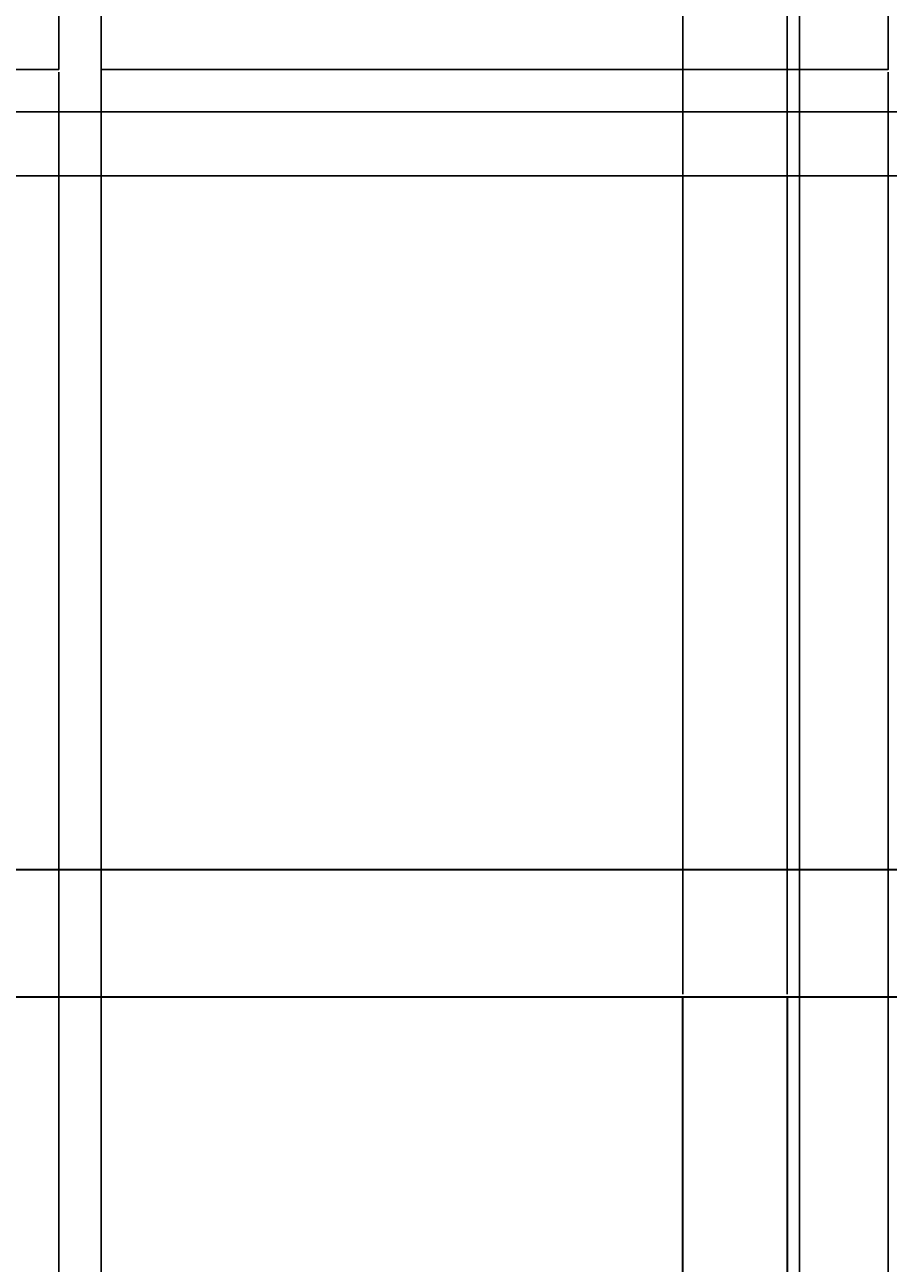
# Model space of a CAD drawing. Units: inches. Extents: x -6 to 289, y -8 to 323.
# Tile 54 of 107: x 146 to 166, y 153 to 182. Entities that reach past the tile are written whole.
import ezdxf

# ---------------------------------------------------------------- set-up
doc = ezdxf.new("R2010")
doc.units = ezdxf.units.IN
doc.header["$MEASUREMENT"] = 0
for name, color, linetype, lineweight in [('A-ANNO-DIMS', 2, 'Continuous', 18), ('A-ELEV', 7, 'Continuous', 35), ('A-ELEV-PATT', 8, 'Continuous', 13), ('A-GLAZ', 4, 'Continuous', 25)]:
    doc.layers.add(name, color=color, linetype=linetype, lineweight=lineweight)
doc.styles.get("Standard").update_dxf_attribs({"font": 'arial.ttf'})
doc.dimstyles.get("Standard").update_dxf_attribs({"dimtxt": 0.18, "dimasz": 0.18, "dimexe": 0.18, "dimexo": 0.0625, "dimgap": 0.09, "dimtad": 0, "dimtih": 1, "dimtoh": 1, "dimdec": 4, "dimzin": 0, "dimdsep": 46, "dimtxsty": 'Standard', "dimcen": 0.09, "dimadec": 0, "dimazin": 0, "dimtfac": 1, "dimtdec": 4, "dimtofl": 0, "dimtmove": 0, "dimatfit": 3, "dimfxl": 1, "dimtolj": 1, "dimtzin": 0, "dimarcsym": 0})

# ---------------------------------------------------------------- blocks, each defined once
blk = doc.blocks.new('*U4')
for p, q in [((21, 1.5), (21, 46.5)), ((21, 1.5), (1.5, 1.5)), ((40.5, 1.5), (21, 1.5))]:
    blk.add_line(p, q)
blk.add_lwpolyline([(0, 0), (0, 48), (42, 48), (42, 0)], close=True)
for points in [[(20, 45.5), (20, 2.5), (2.5, 2.5), (2.5, 45.5), (20, 45.5)], [(21, 45.5), (39.5, 45.5), (39.5, 2.5), (21, 2.5)]]:
    blk.add_lwpolyline(points)
blk = doc.blocks.new('*D24')
at = {"layer": 'A-ANNO-DIMS', "color": 0, "lineweight": -2, "transparency": 16777216}
for p, q in [((126.946, 178.654), (288.653, 178.654)), ((288.473, 178.474), (288.473, 159.153)), ((288.473, 139.469), (288.473, 158.789)), ((259.226, 139.289), (288.653, 139.289))]:
    blk.add_line(p, q, dxfattribs=at)
at = {"layer": 'A-ANNO-DIMS', "color": 0, "transparency": 16777216}
for points in [[(288.443, 178.474), (288.503, 178.474), (288.473, 178.654)], [(288.443, 139.469), (288.503, 139.469), (288.473, 139.289)]]:
    blk.add_solid(points, dxfattribs=at)
at = {"layer": 'Defpoints', "color": 0, "transparency": 16777216}
for p in [(126.883, 178.654), (288.473, 178.654), (259.164, 139.289)]:
    blk.add_point(p, dxfattribs=at)
at = {"layer": 'A-ANNO-DIMS', "color": 0, "transparency": 16777216, "insert": (288.473, 158.971), "char_height": 0.18, "attachment_point": 5}
blk.add_mtext('\\A1;39.365', dxfattribs=at)
blk = doc.blocks.new('*D25')
at = {"layer": 'A-ANNO-DIMS', "color": 0, "lineweight": -2, "transparency": 16777216}
for p, q in [((126.946, 226.654), (288.653, 226.654)), ((288.473, 226.474), (288.473, 202.836)), ((288.473, 178.834), (288.473, 202.472)), ((126.946, 178.654), (288.653, 178.654))]:
    blk.add_line(p, q, dxfattribs=at)
at = {"layer": 'A-ANNO-DIMS', "color": 0, "transparency": 16777216}
for points in [[(288.443, 226.474), (288.503, 226.474), (288.473, 226.654)], [(288.443, 178.834), (288.503, 178.834), (288.473, 178.654)]]:
    blk.add_solid(points, dxfattribs=at)
at = {"layer": 'Defpoints', "color": 0, "transparency": 16777216}
for p in [(126.883, 226.654), (288.473, 226.654), (126.883, 178.654)]:
    blk.add_point(p, dxfattribs=at)
at = {"layer": 'A-ANNO-DIMS', "color": 0, "transparency": 16777216, "insert": (288.473, 202.654), "char_height": 0.18, "attachment_point": 5}
blk.add_mtext('\\A1;48', dxfattribs=at)
blk = doc.blocks.new('*D30')
at = {"layer": 'A-ANNO-DIMS', "color": 0, "lineweight": -2, "transparency": 16777216}
for p, q in [((129.383, 181.092), (129.383, -8.391)), ((146.883, 181.092), (146.883, -8.391)), ((129.563, -8.211), (137.817, -8.211)), ((146.703, -8.211), (138.449, -8.211))]:
    blk.add_line(p, q, dxfattribs=at)
at = {"layer": 'A-ANNO-DIMS', "color": 0, "transparency": 16777216}
for points in [[(129.563, -8.181), (129.563, -8.241), (129.383, -8.211)], [(146.703, -8.181), (146.703, -8.241), (146.883, -8.211)]]:
    blk.add_solid(points, dxfattribs=at)
at = {"layer": 'Defpoints', "color": 0, "transparency": 16777216}
for p in [(129.383, 181.154), (146.883, 181.154), (146.883, -8.211)]:
    blk.add_point(p, dxfattribs=at)
at = {"layer": 'A-ANNO-DIMS', "color": 0, "transparency": 16777216, "insert": (138.133, -8.211), "char_height": 0.18, "attachment_point": 5}
blk.add_mtext('\\A1;17.5', dxfattribs=at)
blk = doc.blocks.new('*D31')
at = {"layer": 'A-ANNO-DIMS', "color": 0, "lineweight": -2, "transparency": 16777216}
for p, q in [((146.883, 181.092), (146.883, -8.391)), ((147.883, 181.092), (147.883, -8.391)), ((147.063, -8.211), (147.26, -8.211)), ((147.703, -8.211), (147.507, -8.211))]:
    blk.add_line(p, q, dxfattribs=at)
at = {"layer": 'A-ANNO-DIMS', "color": 0, "transparency": 16777216}
for points in [[(147.063, -8.181), (147.063, -8.241), (146.883, -8.211)], [(147.703, -8.181), (147.703, -8.241), (147.883, -8.211)]]:
    blk.add_solid(points, dxfattribs=at)
at = {"layer": 'Defpoints', "color": 0, "transparency": 16777216}
for p in [(146.883, 181.154), (147.883, 181.154), (147.883, -8.211)]:
    blk.add_point(p, dxfattribs=at)
at = {"layer": 'A-ANNO-DIMS', "color": 0, "transparency": 16777216, "insert": (147.383, -8.211), "char_height": 0.18, "attachment_point": 5}
blk.add_mtext('\\A1;1', dxfattribs=at)
blk = doc.blocks.new('*D32')
at = {"layer": 'A-ANNO-DIMS', "color": 0, "lineweight": -2, "transparency": 16777216}
for p, q in [((147.883, 181.092), (147.883, -8.391)), ((166.383, 181.092), (166.383, -8.391)), ((148.063, -8.211), (156.817, -8.211)), ((166.203, -8.211), (157.449, -8.211))]:
    blk.add_line(p, q, dxfattribs=at)
at = {"layer": 'A-ANNO-DIMS', "color": 0, "transparency": 16777216}
for points in [[(148.063, -8.181), (148.063, -8.241), (147.883, -8.211)], [(166.203, -8.181), (166.203, -8.241), (166.383, -8.211)]]:
    blk.add_solid(points, dxfattribs=at)
at = {"layer": 'Defpoints', "color": 0, "transparency": 16777216}
for p in [(147.883, 181.154), (166.383, 181.154), (166.383, -8.211)]:
    blk.add_point(p, dxfattribs=at)
at = {"layer": 'A-ANNO-DIMS', "color": 0, "transparency": 16777216, "insert": (157.133, -8.211), "char_height": 0.18, "attachment_point": 5}
blk.add_mtext('\\A1;18.5', dxfattribs=at)
blk = doc.blocks.new('*D76')
at = {"layer": 'A-ANNO-DIMS', "color": 0, "lineweight": -2, "transparency": 16777216}
for p, q in [((142.296, 51.148), (142.296, 322.969)), ((164.296, 51.148), (164.296, 322.969)), ((142.476, 322.789), (153.076, 322.789)), ((164.116, 322.789), (153.516, 322.789))]:
    blk.add_line(p, q, dxfattribs=at)
at = {"layer": 'A-ANNO-DIMS', "color": 0, "transparency": 16777216}
for points in [[(142.476, 322.819), (142.476, 322.759), (142.296, 322.789)], [(164.116, 322.819), (164.116, 322.759), (164.296, 322.789)]]:
    blk.add_solid(points, dxfattribs=at)
at = {"layer": 'Defpoints', "color": 0, "transparency": 16777216}
for p in [(164.296, 322.789), (142.296, 51.085), (164.296, 51.085)]:
    blk.add_point(p, dxfattribs=at)
at = {"layer": 'A-ANNO-DIMS', "color": 0, "transparency": 16777216, "insert": (153.296, 322.789), "char_height": 0.18, "attachment_point": 5}
blk.add_mtext('\\A1;22', dxfattribs=at)
blk = doc.blocks.new('*D77')
at = {"layer": 'A-ANNO-DIMS', "color": 0, "lineweight": -2, "transparency": 16777216}
for p, q in [((164.296, 51.148), (164.296, 322.969)), ((168.296, 51.148), (168.296, 322.969)), ((164.476, 322.789), (166.144, 322.789)), ((168.116, 322.789), (166.448, 322.789))]:
    blk.add_line(p, q, dxfattribs=at)
at = {"layer": 'A-ANNO-DIMS', "color": 0, "transparency": 16777216}
for points in [[(164.476, 322.819), (164.476, 322.759), (164.296, 322.789)], [(168.116, 322.819), (168.116, 322.759), (168.296, 322.789)]]:
    blk.add_solid(points, dxfattribs=at)
at = {"layer": 'Defpoints', "color": 0, "transparency": 16777216}
for p in [(168.296, 322.789), (164.296, 51.085), (168.296, 51.085)]:
    blk.add_point(p, dxfattribs=at)
at = {"layer": 'A-ANNO-DIMS', "color": 0, "transparency": 16777216, "insert": (166.296, 322.789), "char_height": 0.18, "attachment_point": 5}
blk.add_mtext('\\A1;4', dxfattribs=at)
blk = doc.blocks.new('*D94')
at = {"layer": 'A-ANNO-DIMS', "color": 0, "lineweight": -2, "transparency": 16777216}
for p, q in [((118.164, 159.411), (118.164, 322.969)), ((161.552, 159.411), (161.552, 322.969)), ((118.344, 322.789), (139.46, 322.789)), ((161.372, 322.789), (140.256, 322.789))]:
    blk.add_line(p, q, dxfattribs=at)
at = {"layer": 'A-ANNO-DIMS', "color": 0, "transparency": 16777216}
for points in [[(118.344, 322.819), (118.344, 322.759), (118.164, 322.789)], [(161.372, 322.819), (161.372, 322.759), (161.552, 322.789)]]:
    blk.add_solid(points, dxfattribs=at)
at = {"layer": 'Defpoints', "color": 0, "transparency": 16777216}
for p in [(161.552, 322.789), (118.164, 159.348), (161.552, 159.348)]:
    blk.add_point(p, dxfattribs=at)
at = {"layer": 'A-ANNO-DIMS', "color": 0, "transparency": 16777216, "insert": (139.858, 322.789), "char_height": 0.18, "attachment_point": 5}
blk.add_mtext('\\A1;43.39', dxfattribs=at)
blk = doc.blocks.new('*D95')
at = {"layer": 'A-ANNO-DIMS', "color": 0, "lineweight": -2, "transparency": 16777216}
for p, q in [((161.552, 159.411), (161.552, 322.969)), ((164.004, 159.411), (164.004, 322.969)), ((161.732, 322.789), (162.452, 322.789)), ((163.824, 322.789), (163.104, 322.789))]:
    blk.add_line(p, q, dxfattribs=at)
at = {"layer": 'A-ANNO-DIMS', "color": 0, "transparency": 16777216}
for points in [[(161.732, 322.819), (161.732, 322.759), (161.552, 322.789)], [(163.824, 322.819), (163.824, 322.759), (164.004, 322.789)]]:
    blk.add_solid(points, dxfattribs=at)
at = {"layer": 'Defpoints', "color": 0, "transparency": 16777216}
for p in [(164.004, 322.789), (161.552, 159.348), (164.004, 159.348)]:
    blk.add_point(p, dxfattribs=at)
at = {"layer": 'A-ANNO-DIMS', "color": 0, "transparency": 16777216, "insert": (162.778, 322.789), "char_height": 0.18, "attachment_point": 5}
blk.add_mtext('\\A1;2.45', dxfattribs=at)
blk = doc.blocks.new('*D96')
at = {"layer": 'A-ANNO-DIMS', "color": 0, "lineweight": -2, "transparency": 16777216}
for p, q in [((164.004, 159.411), (164.004, 322.969)), ((200.616, 159.411), (200.616, 322.969)), ((164.184, 322.789), (181.934, 322.789)), ((200.436, 322.789), (182.686, 322.789))]:
    blk.add_line(p, q, dxfattribs=at)
at = {"layer": 'A-ANNO-DIMS', "color": 0, "transparency": 16777216}
for points in [[(164.184, 322.819), (164.184, 322.759), (164.004, 322.789)], [(200.436, 322.819), (200.436, 322.759), (200.616, 322.789)]]:
    blk.add_solid(points, dxfattribs=at)
at = {"layer": 'Defpoints', "color": 0, "transparency": 16777216}
for p in [(200.616, 322.789), (164.004, 159.348), (200.616, 159.348)]:
    blk.add_point(p, dxfattribs=at)
at = {"layer": 'A-ANNO-DIMS', "color": 0, "transparency": 16777216, "insert": (182.31, 322.789), "char_height": 0.18, "attachment_point": 5}
blk.add_mtext('\\A1;36.61', dxfattribs=at)

msp = doc.modelspace()

# ---------------------------------------------------------------- hatches: boundary and pattern name
at = {"layer": 'A-ELEV-PATT'}
h = msp.add_hatch(dxfattribs=at)
h.set_pattern_fill('_USER', color=256, scale=6, pattern_type=0)
h.set_pattern_definition([(0, (0, 0), (0, 6), [])])
h.paths.add_polyline_path([(184.1244, 48.0851), (124.008, 48.0851), (124.008, 10.2888), (184.1244, 10.2888)])
h.paths.add_polyline_path([(244.2408, 48.0851), (186.3604, 48.0851), (186.3604, 10.2888), (244.2408, 10.2888)])
h.paths.add_polyline_path([(208.2918, 114.2795), (190.7918, 114.2795), (190.7918, 71.2795), (208.2918, 71.2795)])
h.paths.add_polyline_path([(227.7918, 114.2795), (209.2918, 114.2795), (209.2918, 71.2795), (227.7918, 71.2795)])
h.paths.add_polyline_path([(211.2918, 224.3887), (190.7918, 224.3887), (190.7918, 162.3484), (211.2918, 162.3484)])
h.paths.add_polyline_path([(233.7918, 224.3887), (212.2918, 224.3887), (212.2918, 162.3484), (233.7918, 162.3484)])
h.paths.add_polyline_path([(166.3835, 224.154), (147.8835, 224.154), (147.8835, 181.154), (166.3835, 181.154)])
h.paths.add_polyline_path([(146.8835, 224.154), (129.3835, 224.154), (129.3835, 181.154), (146.8835, 181.154)])

# ---------------------------------------------------------------- linework, layer by layer
at = {"layer": 'A-ELEV'}
for points in [[(247.1638, 139.2888), (115.1638, 139.2888), (115.1638, 162.3484), (247.1638, 162.3484)], [(244.1638, 142.2888), (118.1638, 142.2888), (118.1638, 159.3484), (244.1638, 159.3484)], [(161.5522, 159.3484), (164.0039, 159.3484), (164.0039, 142.2888), (161.5522, 142.2888)]]:
    msp.add_lwpolyline(points, close=True, dxfattribs=at)

# ---------------------------------------------------------------- block references
at = {"layer": 'A-GLAZ'}
msp.add_blockref('*U4', (126.8835, 178.654), dxfattribs=at)

# ---------------------------------------------------------------- dimensions: what is measured, and where the dimension line sits
at = {"layer": 'A-ANNO-DIMS'}
for base, p1, p2, override, picture, middle in [((161.5522, 322.7888), (118.1638, 159.3484), (161.5522, 159.3484), {"dimdec": 2, "dimlfac": 1, "dimrnd": 0, "dimzin": 0, "dimdsep": 46, "dimlunit": 2}, '*D94', (139.858, 322.7888)), ((164.296, 322.7888), (142.296, 51.0851), (164.296, 51.0851), {"dimdec": 0, "dimlfac": 1, "dimrnd": 0, "dimzin": 0, "dimdsep": 46, "dimlunit": 2}, '*D76', (153.296, 322.7888)), ((164.0039, 322.7888), (161.5522, 159.3484), (164.0039, 159.3484), {"dimdec": 2, "dimlfac": 1, "dimrnd": 0, "dimzin": 0, "dimdsep": 46, "dimlunit": 2}, '*D95', (162.7781, 322.7888)), ((200.6162, 322.7888), (164.0039, 159.3484), (200.6162, 159.3484), {"dimdec": 2, "dimlfac": 1, "dimrnd": 0, "dimzin": 0, "dimdsep": 46, "dimlunit": 2}, '*D96', (182.3101, 322.7888)), ((168.296, 322.7888), (164.296, 51.0851), (168.296, 51.0851), {"dimdec": 0, "dimlfac": 1, "dimrnd": 0, "dimzin": 0, "dimdsep": 46, "dimlunit": 2}, '*D77', (166.296, 322.7888)), ((146.8835, -8.2112), (129.3835, 181.154), (146.8835, 181.154), {"dimdec": 1, "dimlfac": 1, "dimrnd": 0, "dimzin": 0, "dimdsep": 46, "dimlunit": 2}, '*D30', (138.1335, -8.2112)), ((147.8835, -8.2112), (146.8835, 181.154), (147.8835, 181.154), {"dimdec": 0, "dimlfac": 1, "dimrnd": 0, "dimzin": 0, "dimdsep": 46, "dimlunit": 2}, '*D31', (147.3835, -8.2112)), ((166.3835, -8.2112), (147.8835, 181.154), (166.3835, 181.154), {"dimdec": 1, "dimlfac": 1, "dimrnd": 0, "dimzin": 0, "dimdsep": 46, "dimlunit": 2}, '*D32', (157.1335, -8.2112))]:
    dim = msp.add_linear_dim(base=base, p1=p1, p2=p2, dimstyle='Standard', override=override, dxfattribs=at)
    dim.commit()
    dim.dimension.update_dxf_attribs({"geometry": picture, "text_midpoint": middle})
for base, p1, p2, override, picture, middle in [((288.4733, 226.654), (126.8835, 178.654), (126.8835, 226.654), {"dimdec": 0, "dimlfac": 1, "dimrnd": 0, "dimzin": 0, "dimdsep": 46, "dimlunit": 2}, '*D25', (288.4733, 202.654)), ((288.4733, 178.654), (259.1638, 139.2888), (126.8835, 178.654), {"dimdec": 3, "dimlfac": 1, "dimrnd": 0, "dimzin": 0, "dimdsep": 46, "dimlunit": 2}, '*D24', (288.4733, 158.9714))]:
    dim = msp.add_linear_dim(base=base, p1=p1, p2=p2, angle=90, dimstyle='Standard', override=override, dxfattribs=at)
    dim.commit()
    dim.dimension.update_dxf_attribs({"geometry": picture, "text_midpoint": middle})

doc.saveas('drawing.dxf')
